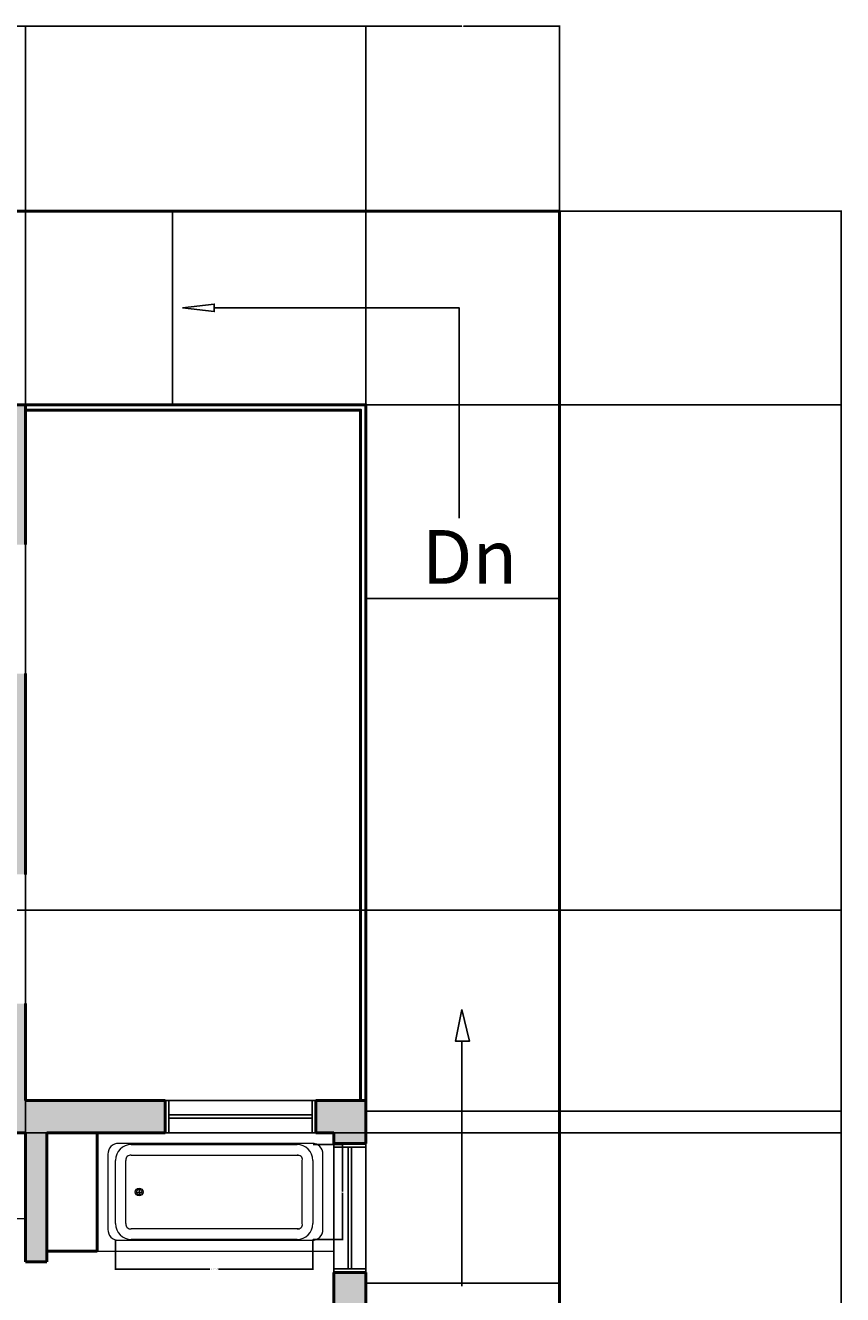
# Model space of a CAD drawing. Units: inches. Extents: x 296 to 2116, y 330 to 1460.
# Tile 6 of 9: x 1008 to 1235, y 1106 to 1460. Entities that reach past the tile are written whole.
import ezdxf

# ---------------------------------------------------------------- set-up
doc = ezdxf.new("R2010")
doc.units = ezdxf.units.IN
for name, color, linetype, lineweight in [('A-ANNO-DIMS', 2, 'Continuous', 18), ('A-ANNO-TEXT', 7, 'Continuous', 18), ('A-FLOR-FIXT', 8, 'Continuous', 18), ('A-FLOR-STRS', 40, 'Continuous', 25), ('A-GLAZ', 4, 'Continuous', 25), ('A-WALL', 7, 'Continuous', 50), ('A-WALL-PATT', 8, 'Continuous', 13)]:
    doc.layers.add(name, color=color, linetype=linetype, lineweight=lineweight)
doc.styles.get("Standard").update_dxf_attribs({"font": 'arial.ttf'})
doc.dimstyles.get("Standard").update_dxf_attribs({"dimtxt": 0.18, "dimasz": 0.18, "dimexe": 0.18, "dimexo": 0.0625, "dimgap": 0.09, "dimtad": 0, "dimtih": 1, "dimtoh": 1, "dimdec": 4, "dimzin": 0, "dimdsep": 46, "dimtxsty": 'Standard', "dimcen": 0.09, "dimadec": 0, "dimazin": 0, "dimtfac": 1, "dimtdec": 4, "dimtofl": 0, "dimtmove": 0, "dimatfit": 3, "dimfxl": 1, "dimtolj": 1, "dimtzin": 0, "dimarcsym": 0})

# ---------------------------------------------------------------- blocks, each defined once
blk = doc.blocks.new('Bath Tub - 26 x 60 in.')
for p, q in [((6, 0), (69, 0)), ((0, -30), (0, -6)), ((75, -6), (75, -30)), ((8, -18), (10, -18)), ((9, -17), (9, -19)), ((69, -36), (6, -36))]:
    blk.add_line(p, q)
for points in [[(6, -4), (69.5, -4)], [(4, -30), (4, -6)], [(71, -30), (71, -6)], [(69.5, -32), (6, -32)]]:
    blk.add_lwpolyline(points)
for radius in [1.5, 1]:
    blk.add_circle((9, -18), radius)
for centre, radius, start, end in [((6, -6), 6, 90, 180), ((69, -6), 6, 0, 90), ((5.75, -5.75), 1.77, 81.8699, 188.1301), ((69.25, -5.75), 1.77, 351.8699, 98.1301), ((6, -30), 6, 180, 270), ((5.75, -30.25), 1.77, 171.8699, 278.1301), ((69.25, -30.25), 1.77, 261.8699, 8.1301), ((69, -30), 6, 270, 0)]:
    blk.add_arc(centre, radius, start, end)
blk = doc.blocks.new('*D39')
at = {"layer": 'A-ANNO-DIMS', "color": 0, "lineweight": -2, "transparency": 16777216}
for p, q in [((1032.65, 1121.13), (1032.65, 1112.75)), ((1087.72, 1121.13), (1087.72, 1112.75)), ((1032.83, 1112.93), (1059, 1112.93)), ((1087.54, 1112.93), (1061.36, 1112.93))]:
    blk.add_line(p, q, dxfattribs=at)
at = {"layer": 'A-ANNO-DIMS', "color": 0, "transparency": 16777216}
for points in [[(1032.83, 1112.96), (1032.83, 1112.9), (1032.65, 1112.93)], [(1087.54, 1112.96), (1087.54, 1112.9), (1087.72, 1112.93)]]:
    blk.add_solid(points, dxfattribs=at)
at = {"layer": 'Defpoints', "color": 0, "transparency": 16777216}
for p in [(1032.65, 1121.19), (1087.72, 1121.19), (1087.72, 1112.93)]:
    blk.add_point(p, dxfattribs=at)
at = {"layer": 'A-ANNO-DIMS', "color": 0, "transparency": 16777216, "insert": (1060.18, 1112.93), "char_height": 0.18, "attachment_point": 5}
blk.add_mtext('\\A1;BATH TUB 55 TYP.', dxfattribs=at)
blk = doc.blocks.new('*D40')
at = {"layer": 'A-ANNO-DIMS', "color": 0, "lineweight": -2, "transparency": 16777216}
for p, q in [((1087.78, 1147.62), (1096.16, 1147.62)), ((1095.98, 1147.44), (1095.98, 1134.59)), ((1095.98, 1121.37), (1095.98, 1134.22)), ((1087.78, 1121.19), (1096.16, 1121.19))]:
    blk.add_line(p, q, dxfattribs=at)
at = {"layer": 'A-ANNO-DIMS', "color": 0, "transparency": 16777216}
for points in [[(1095.95, 1147.44), (1096.01, 1147.44), (1095.98, 1147.62)], [(1095.95, 1121.37), (1096.01, 1121.37), (1095.98, 1121.19)]]:
    blk.add_solid(points, dxfattribs=at)
at = {"layer": 'Defpoints', "color": 0, "transparency": 16777216}
for p in [(1087.72, 1147.62), (1095.98, 1147.62), (1087.72, 1121.19)]:
    blk.add_point(p, dxfattribs=at)
at = {"layer": 'A-ANNO-DIMS', "color": 0, "transparency": 16777216, "insert": (1095.98, 1134.41), "char_height": 0.18, "attachment_point": 5}
blk.add_mtext('\\A1;26 TYP.', dxfattribs=at)
blk = doc.blocks.new('*D45')
at = {"layer": 'A-ANNO-DIMS', "color": 0, "lineweight": -2, "transparency": 16777216}
for p, q in [((1156.58, 1407.95), (1235.3, 1407.95)), ((1235.12, 1407.77), (1235.12, 895.66)), ((1235.12, 383.18), (1235.12, 895.29)), ((609.63, 383), (1235.3, 383))]:
    blk.add_line(p, q, dxfattribs=at)
at = {"layer": 'A-ANNO-DIMS', "color": 0, "transparency": 16777216}
for points in [[(1235.09, 1407.77), (1235.15, 1407.77), (1235.12, 1407.95)], [(1235.09, 383.18), (1235.15, 383.18), (1235.12, 383)]]:
    blk.add_solid(points, dxfattribs=at)
at = {"layer": 'Defpoints', "color": 0, "transparency": 16777216}
for p in [(1156.52, 1407.95), (1235.12, 1407.95), (609.57, 383)]:
    blk.add_point(p, dxfattribs=at)
at = {"layer": 'A-ANNO-DIMS', "color": 0, "transparency": 16777216, "insert": (1235.12, 895.48), "char_height": 0.18, "attachment_point": 5}
blk.add_mtext('\\A1;1025', dxfattribs=at)
blk = doc.blocks.new('*D47')
at = {"layer": 'A-ANNO-DIMS', "color": 0, "lineweight": -2, "transparency": 16777216}
for p, q in [((791.52, 1372.02), (791.52, 1459.73)), ((791.7, 1459.55), (946.75, 1459.55)), ((1102.34, 1459.55), (947.29, 1459.55)), ((1102.52, 1354.02), (1102.52, 1459.73))]:
    blk.add_line(p, q, dxfattribs=at)
at = {"layer": 'A-ANNO-DIMS', "color": 0, "transparency": 16777216}
for points in [[(791.7, 1459.58), (791.7, 1459.52), (791.52, 1459.55)], [(1102.34, 1459.58), (1102.34, 1459.52), (1102.52, 1459.55)]]:
    blk.add_solid(points, dxfattribs=at)
at = {"layer": 'Defpoints', "color": 0, "transparency": 16777216}
for p in [(1102.52, 1459.55), (791.52, 1371.95), (1102.52, 1353.95)]:
    blk.add_point(p, dxfattribs=at)
at = {"layer": 'A-ANNO-DIMS', "color": 0, "transparency": 16777216, "insert": (947.02, 1459.55), "char_height": 0.18, "attachment_point": 5}
blk.add_mtext('\\A1;311', dxfattribs=at)
blk = doc.blocks.new('*D48')
at = {"layer": 'A-ANNO-DIMS', "color": 0, "lineweight": -2, "transparency": 16777216}
for p, q in [((1102.52, 1354.02), (1102.52, 1459.73)), ((1102.7, 1459.55), (1129.3, 1459.55)), ((1156.34, 1459.55), (1129.74, 1459.55)), ((1156.52, 1408.02), (1156.52, 1459.73))]:
    blk.add_line(p, q, dxfattribs=at)
at = {"layer": 'A-ANNO-DIMS', "color": 0, "transparency": 16777216}
for points in [[(1102.7, 1459.58), (1102.7, 1459.52), (1102.52, 1459.55)], [(1156.34, 1459.58), (1156.34, 1459.52), (1156.52, 1459.55)]]:
    blk.add_solid(points, dxfattribs=at)
at = {"layer": 'Defpoints', "color": 0, "transparency": 16777216}
for p in [(1156.52, 1459.55), (1156.52, 1407.95), (1102.52, 1353.95)]:
    blk.add_point(p, dxfattribs=at)
at = {"layer": 'A-ANNO-DIMS', "color": 0, "transparency": 16777216, "insert": (1129.52, 1459.55), "char_height": 0.18, "attachment_point": 5}
blk.add_mtext('\\A1;54', dxfattribs=at)
blk = doc.blocks.new('*D63')
at = {"layer": 'A-ANNO-DIMS', "color": 0, "lineweight": -2, "transparency": 16777216}
for p, q in [((1102.58, 1156.95), (1235.3, 1156.95)), ((1235.12, 1156.77), (1235.12, 973.64)), ((1235.12, 790.13), (1235.12, 973.27)), ((1063.58, 789.95), (1235.3, 789.95))]:
    blk.add_line(p, q, dxfattribs=at)
at = {"layer": 'A-ANNO-DIMS', "color": 0, "transparency": 16777216}
for points in [[(1235.09, 1156.77), (1235.15, 1156.77), (1235.12, 1156.95)], [(1235.09, 790.13), (1235.15, 790.13), (1235.12, 789.95)]]:
    blk.add_solid(points, dxfattribs=at)
at = {"layer": 'Defpoints', "color": 0, "transparency": 16777216}
for p in [(1102.52, 1156.95), (1235.12, 1156.95), (1063.52, 789.95)]:
    blk.add_point(p, dxfattribs=at)
at = {"layer": 'A-ANNO-DIMS', "color": 0, "transparency": 16777216, "insert": (1235.12, 973.45), "char_height": 0.18, "attachment_point": 5}
blk.add_mtext('\\A1;367', dxfattribs=at)
blk = doc.blocks.new('*D64')
at = {"layer": 'A-ANNO-DIMS', "color": 0, "lineweight": -2, "transparency": 16777216}
for p, q in [((1102.58, 1353.95), (1235.3, 1353.95)), ((1235.12, 1353.77), (1235.12, 1255.64)), ((1235.12, 1157.13), (1235.12, 1255.27)), ((1102.58, 1156.95), (1235.3, 1156.95))]:
    blk.add_line(p, q, dxfattribs=at)
at = {"layer": 'A-ANNO-DIMS', "color": 0, "transparency": 16777216}
for points in [[(1235.09, 1353.77), (1235.15, 1353.77), (1235.12, 1353.95)], [(1235.09, 1157.13), (1235.15, 1157.13), (1235.12, 1156.95)]]:
    blk.add_solid(points, dxfattribs=at)
at = {"layer": 'Defpoints', "color": 0, "transparency": 16777216}
for p in [(1102.52, 1353.95), (1235.12, 1353.95), (1102.52, 1156.95)]:
    blk.add_point(p, dxfattribs=at)
at = {"layer": 'A-ANNO-DIMS', "color": 0, "transparency": 16777216, "insert": (1235.12, 1255.45), "char_height": 0.18, "attachment_point": 5}
blk.add_mtext('\\A1;197', dxfattribs=at)
blk = doc.blocks.new('*D65')
at = {"layer": 'A-ANNO-DIMS', "color": 0, "lineweight": -2, "transparency": 16777216}
for p, q in [((1156.58, 1407.95), (1235.3, 1407.95)), ((1235.12, 1407.77), (1235.12, 1381.14)), ((1235.12, 1354.13), (1235.12, 1380.77)), ((1102.58, 1353.95), (1235.3, 1353.95))]:
    blk.add_line(p, q, dxfattribs=at)
at = {"layer": 'A-ANNO-DIMS', "color": 0, "transparency": 16777216}
for points in [[(1235.09, 1407.77), (1235.15, 1407.77), (1235.12, 1407.95)], [(1235.09, 1354.13), (1235.15, 1354.13), (1235.12, 1353.95)]]:
    blk.add_solid(points, dxfattribs=at)
at = {"layer": 'Defpoints', "color": 0, "transparency": 16777216}
for p in [(1156.52, 1407.95), (1235.12, 1407.95), (1102.52, 1353.95)]:
    blk.add_point(p, dxfattribs=at)
at = {"layer": 'A-ANNO-DIMS', "color": 0, "transparency": 16777216, "insert": (1235.12, 1380.95), "char_height": 0.18, "attachment_point": 5}
blk.add_mtext('\\A1;54', dxfattribs=at)
blk = doc.blocks.new('*D81')
at = {"layer": 'A-ANNO-DIMS', "color": 0, "lineweight": -2, "transparency": 16777216}
for p, q in [((919.52, 1115.02), (919.52, 1459.73)), ((919.7, 1459.55), (963.13, 1459.55)), ((1007.34, 1459.55), (963.92, 1459.55)), ((1007.52, 1151.02), (1007.52, 1459.73))]:
    blk.add_line(p, q, dxfattribs=at)
at = {"layer": 'A-ANNO-DIMS', "color": 0, "transparency": 16777216}
for points in [[(919.7, 1459.58), (919.7, 1459.52), (919.52, 1459.55)], [(1007.34, 1459.58), (1007.34, 1459.52), (1007.52, 1459.55)]]:
    blk.add_solid(points, dxfattribs=at)
at = {"layer": 'Defpoints', "color": 0, "transparency": 16777216}
for p in [(1007.52, 1459.55), (1007.52, 1150.95), (919.52, 1114.95)]:
    blk.add_point(p, dxfattribs=at)
at = {"layer": 'A-ANNO-DIMS', "color": 0, "transparency": 16777216, "insert": (963.52, 1459.55), "char_height": 0.18, "attachment_point": 5}
blk.add_mtext('\\A1;88.00', dxfattribs=at)
blk = doc.blocks.new('*D83')
at = {"layer": 'A-ANNO-DIMS', "color": 0, "lineweight": -2, "transparency": 16777216}
for p, q in [((851.58, 1150.95), (1235.3, 1150.95)), ((1235.12, 1150.77), (1235.12, 1109.14)), ((1235.12, 1067.13), (1235.12, 1108.77)), ((851.58, 1066.95), (1235.3, 1066.95))]:
    blk.add_line(p, q, dxfattribs=at)
at = {"layer": 'A-ANNO-DIMS', "color": 0, "transparency": 16777216}
for points in [[(1235.09, 1150.77), (1235.15, 1150.77), (1235.12, 1150.95)], [(1235.09, 1067.13), (1235.15, 1067.13), (1235.12, 1066.95)]]:
    blk.add_solid(points, dxfattribs=at)
at = {"layer": 'Defpoints', "color": 0, "transparency": 16777216}
for p in [(851.52, 1150.95), (1235.12, 1150.95), (851.52, 1066.95)]:
    blk.add_point(p, dxfattribs=at)
at = {"layer": 'A-ANNO-DIMS', "color": 0, "transparency": 16777216, "insert": (1235.12, 1108.95), "char_height": 0.18, "attachment_point": 5}
blk.add_mtext('\\A1;84.00', dxfattribs=at)
blk = doc.blocks.new('*D85')
at = {"layer": 'A-ANNO-DIMS', "color": 0, "lineweight": -2, "transparency": 16777216}
for p, q in [((788.58, 1213), (1235.3, 1213)), ((1235.12, 1212.82), (1235.12, 1075.18)), ((1235.12, 937.18), (1235.12, 1074.82)), ((788.58, 937), (1235.3, 937))]:
    blk.add_line(p, q, dxfattribs=at)
at = {"layer": 'A-ANNO-DIMS', "color": 0, "transparency": 16777216}
for points in [[(1235.09, 1212.82), (1235.15, 1212.82), (1235.12, 1213)], [(1235.09, 937.18), (1235.15, 937.18), (1235.12, 937)]]:
    blk.add_solid(points, dxfattribs=at)
at = {"layer": 'Defpoints', "color": 0, "transparency": 16777216}
for p in [(788.52, 1213), (1235.12, 1213), (788.52, 937)]:
    blk.add_point(p, dxfattribs=at)
at = {"layer": 'A-ANNO-DIMS', "color": 0, "transparency": 16777216, "insert": (1235.12, 1075), "char_height": 0.18, "attachment_point": 5}
blk.add_mtext('\\A1;276.00', dxfattribs=at)

msp = doc.modelspace()

# ---------------------------------------------------------------- hatches: boundary and pattern name
at = {"layer": 'A-WALL-PATT'}
h = msp.add_hatch(color=256, dxfattribs=at)
h.dxf.hatch_style = 1
h.paths.add_polyline_path([(656.5723, 927.9991), (668.5723, 927.9991), (668.5723, 936.9991), (650.5723, 936.9991), (650.5723, 897.9991), (356.5223, 897.9991), (356.5223, 955.9991), (347.5223, 955.9991), (347.5223, 888.9991), (423.5723, 888.9991), (423.5723, 766.9991), (432.5723, 766.9991), (432.5723, 834.9991), (453.5723, 834.9991), (468.5723, 834.9991), (468.5723, 840.9991), (432.5723, 840.9991), (432.5723, 888.9991), (504.5723, 888.9991), (504.5723, 840.9991), (504.5723, 834.9991), (531.6223, 834.9991), (531.6223, 768.5344), (527.8443, 764.7564), (530.6728, 761.928), (532.087, 760.5138), (540.5723, 768.9991), (598.0723, 768.9991), (598.0723, 777.9991), (601.8223, 777.9991), (601.8223, 782.1991), (601.8223, 783.9991), (598.0723, 783.9991), (598.0723, 798.9991), (592.0723, 798.9991), (592.0723, 774.9991), (537.6223, 774.9991), (537.6223, 834.9991), (592.0723, 834.9991), (592.0723, 828.9991), (598.0723, 828.9991), (598.0723, 834.9991), (647.5723, 834.9991), (647.5723, 828.9991), (656.5723, 828.9991), (656.5723, 846.9991), (650.5723, 846.9991), (647.5723, 846.9991), (647.5723, 840.9991), (510.5723, 840.9991), (510.5723, 888.9991), (647.5723, 888.9991), (647.5723, 882.9991), (656.5723, 882.9991)])
h.paths.add_polyline_path([(432.5723, 730.9991), (496.5723, 730.9991), (496.5723, 724.9991), (502.5723, 724.9991), (502.5723, 730.9991), (506.6311, 735.058), (502.3885, 739.3006), (500.087, 736.9991), (432.5723, 736.9991), (432.5723, 742.9991), (423.5723, 742.9991), (423.5723, 641.9991), (490.5723, 641.9991), (490.5723, 597.9991), (531.5723, 597.9991), (531.5723, 606.9991), (499.5723, 606.9991), (499.5723, 650.9991), (502.5723, 650.9991), (502.5723, 659.9991), (496.5723, 659.9991), (493.5723, 659.9991), (493.5723, 650.9991), (432.5723, 650.9991)])
h.paths.add_polyline_path([(656.5723, 689.4991), (662.5473, 689.4991), (662.5473, 698.4991), (656.5723, 698.4991), (656.5723, 789.9991), (647.5723, 789.9991), (647.5723, 783.9991), (643.8223, 783.9991), (643.8223, 777.9991), (647.5723, 777.9991), (647.5723, 606.9991), (615.5723, 606.9991), (615.5723, 597.9991), (656.5723, 597.9991)])
h.paths.add_polyline_path([(761.5223, 780.9541), (797.5223, 780.9541), (797.5223, 789.9541), (761.5223, 789.9541), (761.5223, 858.9541), (797.5223, 858.9541), (797.5223, 867.9541), (752.5223, 867.9541), (752.5223, 698.4991), (746.5473, 698.4991), (746.5473, 694.2991), (746.5473, 689.4991), (752.5223, 689.4991), (752.5223, 624.9541), (761.5223, 624.9541)])
h.paths.add_polyline_path([(1102.5223, 795.9541), (1093.5223, 795.9541), (1093.5223, 789.9541), (1063.5223, 789.9541), (881.5223, 789.9541), (881.5223, 837.9541), (911.5223, 837.9541), (911.5223, 849.9541), (907.5223, 849.9541), (905.5223, 849.9541), (905.5223, 843.9541), (845.5223, 843.9541), (845.5223, 834.9541), (849.0223, 834.9541), (851.5223, 834.9541), (851.5223, 837.9541), (875.5223, 837.9541), (875.5223, 789.9541), (851.5223, 789.9541), (851.5223, 792.9541), (845.5223, 792.9541), (845.5223, 789.9541), (833.5223, 789.9541), (833.5223, 785.1541), (833.5223, 780.9541), (1049.5223, 780.9541), (1049.5223, 726.9541), (1053.7223, 726.9541), (1058.5223, 726.9541), (1058.5223, 780.9541), (1102.5223, 780.9541)])
h.paths.add_polyline_path([(761.5223, 588.9541), (752.5223, 588.9541), (752.5223, 564.9541), (761.5223, 564.9541)])
h.paths.add_polyline_path([(809.5223, 480.9541), (761.5223, 480.9541), (761.5223, 528.9541), (752.5223, 528.9541), (752.5223, 471.9541), (809.5223, 471.9541)])
h.paths.add_polyline_path([(1058.5223, 684.9541), (1049.5223, 684.9541), (1049.5223, 480.9541), (1001.5223, 480.9541), (1001.5223, 476.4541), (1001.5223, 471.9541), (1058.5223, 471.9541)])
h.paths.add_polyline_path([(794.5223, 1013.9991), (800.5223, 1013.9991), (800.5223, 1019.9991), (794.5223, 1019.9991), (794.5223, 1296.9541), (785.5223, 1296.9541), (785.5223, 1221.9991), (752.5223, 1221.9991), (752.5223, 1212.9991), (788.5223, 1212.9991), (788.5223, 936.9991), (752.5223, 936.9991), (752.5223, 927.9991), (794.5223, 927.9991)])
h.paths.add_polyline_path([(450.0223, 1191.9991), (398.5223, 1191.9991), (398.5223, 1137.9991), (407.5223, 1137.9991), (407.5223, 1182.9991), (450.0223, 1182.9991)])
h.paths.add_polyline_path([(576.5223, 1212.9991), (612.5223, 1212.9991), (612.5223, 1221.9991), (567.5223, 1221.9991), (567.5223, 1191.9991), (540.0223, 1191.9991), (540.0223, 1182.9991), (576.5223, 1182.9991)])
h.paths.add_polyline_path([(407.5223, 1060.9991), (398.5223, 1060.9991), (398.5223, 1030.9991), (392.5223, 1030.9991), (392.5223, 1021.9991), (407.5223, 1021.9991)])
h.paths.add_polyline_path([(356.5223, 1030.9991), (347.5223, 1030.9991), (347.5223, 1015.9991), (356.5223, 1015.9991), (356.5223, 1021.9991)])
h.paths.add_polyline_path([(788.5223, 1129.9991), (770.0334, 1131.3572, 0.43585667), (767.8869, 1129.3626), (767.8869, 1108.3618, 0.31855172), (769.8942, 1105.5308), (788.5223, 1098.9991)], flags=17)
h.paths.add_polyline_path([(788.5223, 1050.9991), (769.8942, 1044.4674, 0.31855172), (767.8869, 1041.6364), (767.8869, 1020.6356, 0.43585667), (770.0334, 1018.641), (788.5223, 1019.9991)], flags=17)
h.paths.add_polyline_path([(893.5223, 1066.9541), (851.5223, 1066.9541), (851.5223, 1069.9541), (845.5223, 1069.9541), (845.5223, 1019.9991), (839.5223, 1019.9991), (839.5223, 1013.9991), (845.5223, 1013.9991), (845.5223, 891.9541), (863.5223, 891.9541), (863.5223, 897.9541), (851.5223, 897.9541), (851.5223, 927.9541), (905.5223, 927.9541), (905.5223, 897.9541), (893.5223, 897.9541), (893.5223, 891.9541), (905.5223, 891.9541), (905.5223, 885.9541), (911.5223, 885.9541), (911.5223, 927.9541), (1030.5223, 927.9541), (1030.5223, 936.9541), (1013.5223, 936.9541), (1013.5223, 996.9541), (1093.5223, 996.9541), (1093.5223, 936.9541), (1066.5223, 936.9541), (1066.5223, 927.9541), (1093.5223, 927.9541), (1093.5223, 921.9541), (1102.5223, 921.9541), (1102.5223, 1013.9541), (1093.5223, 1013.9541), (1093.5223, 1002.9541), (1013.5223, 1002.9541), (1013.5223, 1060.9541), (1013.5223, 1066.9541), (1007.5223, 1066.9541), (1007.5223, 1042.9541), (977.5223, 1042.9541), (977.5223, 1066.9541), (965.5223, 1066.9541), (965.5223, 1060.9541), (971.5223, 1060.9541), (971.5223, 1036.9541), (1007.5223, 1036.9541), (1007.5223, 936.9541), (851.5223, 936.9541), (851.5223, 1060.9541), (893.5223, 1060.9541)])
h.paths.add_polyline_path([(851.5223, 1150.9541), (919.5223, 1150.9541), (919.5223, 1114.9541), (911.5223, 1114.9541), (911.5223, 1108.9541), (925.5223, 1108.9541), (925.5223, 1150.9541), (1007.5223, 1150.9541), (1007.5223, 1114.9541), (1013.5223, 1114.9541), (1013.5223, 1150.9541), (1046.5223, 1150.9541), (1046.5223, 1159.9541), (1007.5223, 1159.9541), (1007.5223, 1186.9541), (998.5223, 1186.9541), (998.5223, 1156.9541), (845.5223, 1156.9541), (845.5223, 1105.9541), (851.5223, 1105.9541)])
h.paths.add_polyline_path([(1102.5223, 1156.9541), (1102.5223, 1159.9541), (1088.5223, 1159.9541), (1088.5223, 1150.9541), (1093.5223, 1150.9541), (1093.5223, 1147.9541), (1102.5223, 1147.9541)])
h.paths.add_polyline_path([(1102.5223, 1111.9541), (1093.5223, 1111.9541), (1093.5223, 1066.9541), (1047.5223, 1066.9541), (1047.5223, 1030.9541), (1053.5223, 1030.9541), (1053.5223, 1060.9541), (1093.5223, 1060.9541), (1093.5223, 1049.9541), (1102.5223, 1049.9541)])
h.paths.add_polyline_path([(1102.5223, 837.9541), (1093.5223, 837.9541), (1093.5223, 831.9541), (1102.5223, 831.9541)], flags=17)
h.paths.add_polyline_path([(1102.5223, 879.9541), (1093.5223, 879.9541), (1093.5223, 873.9541), (1102.5223, 873.9541)])
h.paths.add_polyline_path([(839.5223, 1353.9541), (785.5223, 1353.9541), (785.5223, 1338.9541), (794.5223, 1338.9541), (794.5223, 1344.9541), (839.5223, 1344.9541)])
h.paths.add_polyline_path([(1007.5223, 1353.9541), (953.5223, 1353.9541), (953.5223, 1344.9541), (998.5223, 1344.9541), (998.5223, 1314.9541), (1007.5223, 1314.9541)])
h.paths.add_polyline_path([(917.5223, 1353.9541), (914.5223, 1353.9541), (914.5223, 1344.9541), (917.5223, 1344.9541)])
h.paths.add_polyline_path([(878.5223, 1353.9541), (875.5223, 1353.9541), (875.5223, 1344.9541), (878.5223, 1344.9541)])
h.paths.add_polyline_path([(1007.5223, 1278.9541), (998.5223, 1278.9541), (998.5223, 1222.9541), (1007.5223, 1222.9541)])
h.paths.add_polyline_path([(407.5223, 1101.9991), (398.5223, 1101.9991), (398.5223, 1096.9991), (407.5223, 1096.9991)])
h.paths.add_polyline_path([(560.5723, 606.9991), (557.5723, 606.9991), (557.5723, 597.9991), (560.5723, 597.9991)])
h.paths.add_polyline_path([(589.5723, 606.9991), (586.5723, 606.9991), (586.5723, 597.9991), (589.5723, 597.9991)])

# ---------------------------------------------------------------- linework, layer by layer
at = {"layer": 'A-FLOR-FIXT'}
msp.add_line((1007.5223, 1126.9541), (925.5223, 1126.9541), dxfattribs=at)
msp.add_lwpolyline([(1093.5223, 1150.9541), (1027.5223, 1150.9541), (1027.5223, 1117.9541), (1093.5223, 1117.9541)], close=True, dxfattribs=at)
msp.add_lwpolyline([(1087.5223, 1147.9541), (1033.5223, 1147.9541, 0.41421356), (1030.5223, 1144.9541), (1030.5223, 1123.9541, 0.41421356), (1033.5223, 1120.9541), (1087.5223, 1120.9541, 0.41421356), (1090.5223, 1123.9541), (1090.5223, 1144.9541, 0.41421356)], format="xyb", close=True, dxfattribs=at)
at = {"layer": 'A-FLOR-STRS'}
for p, q in [((1048.5223, 1353.9541), (1048.5223, 1407.9541)), ((1102.5223, 1353.9541), (1102.5223, 1407.9541)), ((1102.5223, 1353.9541), (1156.5223, 1353.9541)), ((1102.5223, 1299.9541), (1156.5223, 1299.9541)), ((1102.5223, 1156.9541), (1156.5223, 1156.9541)), ((1102.5223, 1108.9541), (1156.5223, 1108.9541))]:
    msp.add_line(p, q, dxfattribs=at)
for points in [[(1051.3363, 1380.9541), (1060.2042, 1379.9381), (1060.2042, 1381.9957)], [(1129.2577, 1185.3214), (1131.4027, 1176.4535), (1127.5095, 1176.4535)]]:
    msp.add_lwpolyline(points, close=True, dxfattribs=at)
for points in [[(1128.5448, 1322.3403), (1128.5448, 1380.9541), (1060.2042, 1380.9541)], [(1129.2577, 1108.1129), (1129.2577, 1176.4535)]]:
    msp.add_lwpolyline(points, dxfattribs=at)
at = {"layer": 'A-GLAZ'}
for p, q in [((1047.5223, 1155.9541), (1087.5223, 1155.9541)), ((1047.5223, 1154.9541), (1087.5223, 1154.9541)), ((1093.5223, 1146.9541), (1102.5223, 1146.9541)), ((1097.5223, 1112.9541), (1097.5223, 1146.9541)), ((1098.5223, 1146.9541), (1098.5223, 1112.9541)), ((1102.5223, 1112.9541), (1093.5223, 1112.9541))]:
    msp.add_line(p, q, dxfattribs=at)
for points in [[(1046.5223, 1159.9541), (1088.5223, 1159.9541), (1088.5223, 1150.9541), (1046.5223, 1150.9541)], [(1102.5223, 1111.9541), (1093.5223, 1111.9541), (1093.5223, 1147.9541), (1102.5223, 1147.9541)]]:
    msp.add_lwpolyline(points, close=True, dxfattribs=at)
for points in [[(1047.5223, 1150.9541), (1047.5223, 1159.9541)], [(1087.5223, 1159.9541), (1087.5223, 1150.9541)]]:
    msp.add_lwpolyline(points, dxfattribs=at)
at = {"layer": 'A-WALL'}
for p, q in [((940.5223, 1407.9541), (1156.5223, 1407.9541)), ((1156.5223, 576.9541), (1156.5223, 1407.9541)), ((1007.5223, 1353.9541), (940.5223, 1353.9541)), ((1007.5223, 1314.9541), (1007.5223, 1353.9541)), ((1007.5223, 1222.9541), (1007.5223, 1278.9541)), ((1007.5223, 1159.9541), (1007.5223, 1186.9541)), ((1046.5223, 1150.9541), (1046.5223, 1159.9541)), ((1088.5223, 1150.9541), (1088.5223, 1159.9541)), ((1102.5223, 1159.9541), (1088.5223, 1159.9541)), ((1102.5223, 1147.9541), (1102.5223, 1156.9541)), ((1007.5223, 1150.9541), (925.5223, 1150.9541)), ((1007.5223, 1114.9541), (1007.5223, 1150.9541)), ((1013.5223, 1114.9541), (1013.5223, 1150.9541)), ((1046.5223, 1150.9541), (1013.5223, 1150.9541)), ((1027.5223, 1117.9541), (1027.5223, 1150.9541)), ((1093.5223, 1150.9541), (1088.5223, 1150.9541)), ((1093.5223, 1147.9541), (1093.5223, 1150.9541)), ((1093.5223, 1147.9541), (1102.5223, 1147.9541)), ((1007.5223, 1114.9541), (1013.5223, 1114.9541)), ((1027.5223, 1117.9541), (1013.5223, 1117.9541)), ((1093.5223, 1066.9541), (1093.5223, 1111.9541)), ((1093.5223, 1111.9541), (1102.5223, 1111.9541)), ((1102.5223, 1049.9541), (1102.5223, 1111.9541))]:
    msp.add_line(p, q, dxfattribs=at)
for points in [[(1007.5223, 1353.9541), (1102.5223, 1353.9541), (1102.5223, 1156.9541)], [(1007.5223, 1352.4541), (1101.0223, 1352.4541), (1101.0223, 1159.9541)], [(1046.5223, 1159.9541), (1007.5223, 1159.9541)]]:
    msp.add_lwpolyline(points, dxfattribs=at)

# ---------------------------------------------------------------- block references
at = {"layer": 'A-FLOR-FIXT', "xscale": 0.7342715882899387, "yscale": 0.7342715882899387, "zscale": 0.7342715882899387}
msp.add_blockref('Bath Tub - 26 x 60 in.', (1032.6456, 1147.6232), dxfattribs=at)

# ---------------------------------------------------------------- texts
at = {"layer": 'A-ANNO-TEXT', "insert": (1118.1558, 1319.0076), "char_height": 15, "attachment_point": 1}
msp.add_mtext_dynamic_manual_height_columns('{\\fArial|b1|i0|c0|p34;Dn}', width=22.506546, gutter_width=12.5, heights=[0], dxfattribs=at)

# ---------------------------------------------------------------- dimensions: what is measured, and where the dimension line sits
at = {"layer": 'A-ANNO-DIMS'}
for base, p1, p2, override, picture, middle in [((1102.5223, 1459.5541), (791.5223, 1371.9541), (1102.5223, 1353.9541), {"dimdec": 0, "dimlfac": 1, "dimrnd": 0, "dimzin": 0, "dimdsep": 46, "dimlunit": 2}, '*D47', (947.0223, 1459.5541)), ((1007.5223, 1459.5541), (919.5223, 1114.9541), (1007.5223, 1150.9541), {"dimdec": 2, "dimlfac": 1, "dimrnd": 0, "dimzin": 0, "dimdsep": 46, "dimlunit": 2}, '*D81', (963.5223, 1459.5541)), ((1156.5223, 1459.5541), (1102.5223, 1353.9541), (1156.5223, 1407.9541), {"dimdec": 0, "dimlfac": 1, "dimrnd": 0, "dimzin": 0, "dimdsep": 46, "dimlunit": 2}, '*D48', (1129.5223, 1459.5541))]:
    dim = msp.add_linear_dim(base=base, p1=p1, p2=p2, dimstyle='Standard', override=override, dxfattribs=at)
    dim.commit()
    dim.dimension.update_dxf_attribs({"geometry": picture, "text_midpoint": middle})
for base, p1, p2, override, picture, middle in [((1235.1223, 1407.9541), (609.5723, 382.9991), (1156.5223, 1407.9541), {"dimdec": 0, "dimlfac": 1, "dimrnd": 0, "dimzin": 0, "dimdsep": 46, "dimlunit": 2}, '*D45', (1235.1223, 895.4766)), ((1235.1223, 1407.9541), (1102.5223, 1353.9541), (1156.5223, 1407.9541), {"dimdec": 0, "dimlfac": 1, "dimrnd": 0, "dimzin": 0, "dimdsep": 46, "dimlunit": 2}, '*D65', (1235.1223, 1380.9541)), ((1235.1223, 1353.9541), (1102.5223, 1156.9541), (1102.5223, 1353.9541), {"dimdec": 0, "dimlfac": 1, "dimrnd": 0, "dimzin": 0, "dimdsep": 46, "dimlunit": 2}, '*D64', (1235.1223, 1255.4541)), ((1235.1223, 1212.9991), (788.5223, 936.9991), (788.5223, 1212.9991), {"dimdec": 2, "dimlfac": 1, "dimrnd": 0, "dimzin": 0, "dimdsep": 46, "dimlunit": 2}, '*D85', (1235.1223, 1074.9991)), ((1235.1223, 1156.9541), (1063.5223, 789.9541), (1102.5223, 1156.9541), {"dimdec": 0, "dimlfac": 1, "dimrnd": 0, "dimzin": 0, "dimdsep": 46, "dimlunit": 2}, '*D63', (1235.1223, 973.4541)), ((1235.1223, 1150.9541), (851.5223, 1066.9541), (851.5223, 1150.9541), {"dimdec": 2, "dimlfac": 1, "dimrnd": 0, "dimzin": 0, "dimdsep": 46, "dimlunit": 2}, '*D83', (1235.1223, 1108.9541))]:
    dim = msp.add_linear_dim(base=base, p1=p1, p2=p2, angle=90, dimstyle='Standard', override=override, dxfattribs=at)
    dim.commit()
    dim.dimension.update_dxf_attribs({"geometry": picture, "text_midpoint": middle})
dim = msp.add_linear_dim(base=(1095.9766, 1147.6232), p1=(1087.716, 1121.1894), p2=(1087.716, 1147.6232), angle=90, text='<> TYP.', dimstyle='Standard', override={"dimdec": 0, "dimrnd": 0, "dimzin": 0, "dimlunit": 2}, dxfattribs=at)
dim.commit()
dim.dimension.update_dxf_attribs({"geometry": '*D40', "text_midpoint": (1095.9766, 1134.4063)})
dim = msp.add_linear_dim(base=(1087.716, 1112.9288), p1=(1032.6456, 1121.1894), p2=(1087.716, 1121.1894), text='BATH TUB <> TYP.', dimstyle='Standard', override={"dimdec": 0, "dimrnd": 0, "dimzin": 0, "dimlunit": 2}, dxfattribs=at)
dim.commit()
dim.dimension.update_dxf_attribs({"geometry": '*D39', "text_midpoint": (1060.1808, 1112.9288)})

doc.saveas('drawing.dxf')
